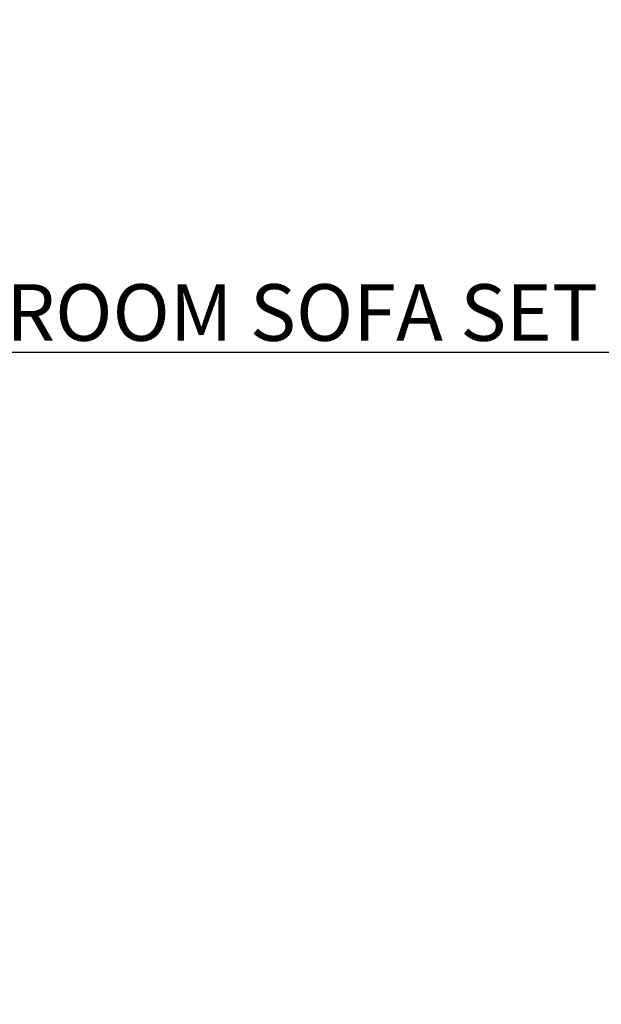
# Model space of a CAD drawing. Units: inches. Extents: x 261 to 2725, y 291 to 1454.
# Tile 18 of 35: x 1043 to 1166, y 644 to 853. Entities that reach past the tile are written whole.
import ezdxf

# ---------------------------------------------------------------- set-up
doc = ezdxf.new("R2010")
doc.units = ezdxf.units.IN
doc.layers.add('A-ANNO-DIMS', color=136, linetype='Continuous', lineweight=18)
doc.styles.get("Standard").update_dxf_attribs({"font": 'arial.ttf'})
doc.dimstyles.new('ISO-25', dxfattribs={"dimtxt": 12, "dimasz": 6, "dimexe": 1.25, "dimexo": 0.625, "dimtad": 1, "dimdec": 0, "dimlunit": 3, "dimtxsty": 'Standard', "dimblk": 'ARCHTICK', "dimcen": 2.5, "dimadec": 0, "dimazin": 0, "dimtfac": 1, "dimtdec": 0, "dimtmove": 0, "dimatfit": 3, "dimfxl": 1, "dimfxlon": 1, "dimarcsym": 0})

# ---------------------------------------------------------------- blocks, each defined once
blk = doc.blocks.new('_ArchTick')
at = {"color": 0, "linetype": 'ByBlock', "const_width": 0.15}
blk.add_lwpolyline([(-0.5, -0.5), (0.5, 0.5)], dxfattribs=at)
blk = doc.blocks.new('*D69')
at = {"layer": 'A-ANNO-DIMS', "color": 0, "lineweight": -2, "ltscale": 0.07, "transparency": 16777216}
for p, q in [((772.63, 783.4), (772.63, 781.15)), ((946.45, 783.4), (946.45, 781.15)), ((772.63, 782.4), (946.45, 782.4)), ((946.45, 782.4), (1224.37, 782.4))]:
    blk.add_line(p, q, dxfattribs=at)
at = {"layer": 'Defpoints', "color": 0, "ltscale": 0.07, "transparency": 16777216}
for p in [(772.63, 808.47), (946.45, 808.47), (946.45, 782.4)]:
    blk.add_point(p, dxfattribs=at)
at = {"layer": 'A-ANNO-DIMS', "color": 0, "lineweight": -2, "ltscale": 0.07, "transparency": 16777216, "xscale": 6, "yscale": 6, "zscale": 6, "rotation": 180}
blk.add_blockref('_ArchTick', (772.63, 782.4), dxfattribs=at)
at = {"layer": 'A-ANNO-DIMS', "color": 0, "lineweight": -2, "ltscale": 0.07, "transparency": 16777216, "xscale": 6, "yscale": 6, "zscale": 6}
blk.add_blockref('_ArchTick', (946.45, 782.4), dxfattribs=at)
at = {"layer": 'A-ANNO-DIMS', "color": 0, "ltscale": 0.07, "transparency": 16777216, "insert": (1088.41, 789.23), "char_height": 12, "attachment_point": 5}
blk.add_mtext('DRAWING ROOM SOFA SET 14\'-6"', dxfattribs=at)
blk = doc.blocks.new('*D82')
at = {"layer": 'A-ANNO-DIMS', "color": 0, "lineweight": -2, "ltscale": 0.07, "transparency": 16777216}
for p, q in [((2600.96, 679.47), (2603.21, 679.47)), ((2601.96, 517.47), (2601.96, 679.47)), ((2600.96, 517.47), (2603.21, 517.47))]:
    blk.add_line(p, q, dxfattribs=at)
at = {"layer": 'Defpoints', "color": 0, "ltscale": 0.07, "transparency": 16777216}
for p in [(946.45, 679.47), (2601.96, 679.47), (946.45, 517.47)]:
    blk.add_point(p, dxfattribs=at)
at = {"layer": 'A-ANNO-DIMS', "color": 0, "lineweight": -2, "ltscale": 0.07, "transparency": 16777216, "xscale": 6, "yscale": 6, "zscale": 6}
for p, rotation in [((2601.96, 679.47), 90), ((2601.96, 517.47), 270)]:
    blk.add_blockref('_ArchTick', p, dxfattribs=dict(at, rotation=rotation))
at = {"layer": 'A-ANNO-DIMS', "color": 0, "ltscale": 0.07, "transparency": 16777216, "insert": (2595.2, 598.47), "char_height": 12, "attachment_point": 5, "rotation": 90}
blk.add_mtext('13\'-6"', dxfattribs=at)
blk = doc.blocks.new('*D83')
at = {"layer": 'A-ANNO-DIMS', "color": 0, "lineweight": -2, "ltscale": 0.07, "transparency": 16777216}
for p, q in [((2600.96, 799.47), (2603.21, 799.47)), ((2601.96, 679.47), (2601.96, 799.47)), ((2600.96, 679.47), (2603.21, 679.47))]:
    blk.add_line(p, q, dxfattribs=at)
at = {"layer": 'Defpoints', "color": 0, "ltscale": 0.07, "transparency": 16777216}
for p in [(946.45, 799.47), (2601.96, 799.47), (946.45, 679.47)]:
    blk.add_point(p, dxfattribs=at)
at = {"layer": 'A-ANNO-DIMS', "color": 0, "lineweight": -2, "ltscale": 0.07, "transparency": 16777216, "xscale": 6, "yscale": 6, "zscale": 6}
for p, rotation in [((2601.96, 799.47), 90), ((2601.96, 679.47), 270)]:
    blk.add_blockref('_ArchTick', p, dxfattribs=dict(at, rotation=rotation))
at = {"layer": 'A-ANNO-DIMS', "color": 0, "ltscale": 0.07, "transparency": 16777216, "insert": (2595.21, 739.47), "char_height": 12, "attachment_point": 5, "rotation": 90}
blk.add_mtext('10\'-0"', dxfattribs=at)
blk = doc.blocks.new('*D84')
at = {"layer": 'A-ANNO-DIMS', "color": 0, "lineweight": -2, "ltscale": 0.07, "transparency": 16777216}
for p, q in [((2600.96, 1024.47), (2603.21, 1024.47)), ((2601.96, 799.47), (2601.96, 1024.47)), ((2600.96, 799.47), (2603.21, 799.47))]:
    blk.add_line(p, q, dxfattribs=at)
at = {"layer": 'Defpoints', "color": 0, "ltscale": 0.07, "transparency": 16777216}
for p in [(946.45, 1024.47), (2601.96, 1024.47), (946.45, 799.47)]:
    blk.add_point(p, dxfattribs=at)
at = {"layer": 'A-ANNO-DIMS', "color": 0, "lineweight": -2, "ltscale": 0.07, "transparency": 16777216, "xscale": 6, "yscale": 6, "zscale": 6}
for p, rotation in [((2601.96, 1024.47), 90), ((2601.96, 799.47), 270)]:
    blk.add_blockref('_ArchTick', p, dxfattribs=dict(at, rotation=rotation))
at = {"layer": 'A-ANNO-DIMS', "color": 0, "ltscale": 0.07, "transparency": 16777216, "insert": (2595.21, 911.97), "char_height": 12, "attachment_point": 5, "rotation": 90}
blk.add_mtext('18\'-9"', dxfattribs=at)
blk = doc.blocks.new('*D103')
at = {"layer": 'A-ANNO-DIMS', "color": 0, "lineweight": -2, "ltscale": 0.07, "transparency": 16777216}
for p, q in [((287.06, 1231.47), (284.81, 1231.47)), ((286.06, 439.47), (286.06, 1231.47)), ((287.06, 439.47), (284.81, 439.47))]:
    blk.add_line(p, q, dxfattribs=at)
at = {"layer": 'Defpoints', "color": 0, "ltscale": 0.07, "transparency": 16777216}
for p in [(286.06, 1231.47), (1243.08, 1231.47), (1243.08, 439.47)]:
    blk.add_point(p, dxfattribs=at)
at = {"layer": 'A-ANNO-DIMS', "color": 0, "lineweight": -2, "ltscale": 0.07, "transparency": 16777216, "xscale": 6, "yscale": 6, "zscale": 6}
for p, rotation in [((286.06, 1231.47), 90), ((286.06, 439.47), 270)]:
    blk.add_blockref('_ArchTick', p, dxfattribs=dict(at, rotation=rotation))
at = {"layer": 'A-ANNO-DIMS', "color": 0, "ltscale": 0.07, "transparency": 16777216, "insert": (279.3, 835.47), "char_height": 12, "attachment_point": 5, "rotation": 90}
blk.add_mtext('66\'-0"', dxfattribs=at)
blk = doc.blocks.new('*D107')
at = {"layer": 'A-ANNO-DIMS', "color": 0, "lineweight": -2, "ltscale": 0.07, "transparency": 16777216}
for p, q in [((287.06, 673.47), (284.81, 673.47)), ((286.06, 496.47), (286.06, 673.47)), ((287.06, 496.47), (284.81, 496.47))]:
    blk.add_line(p, q, dxfattribs=at)
at = {"layer": 'Defpoints', "color": 0, "ltscale": 0.07, "transparency": 16777216}
for p in [(286.06, 673.47), (1252.08, 673.47), (1252.08, 496.47)]:
    blk.add_point(p, dxfattribs=at)
at = {"layer": 'A-ANNO-DIMS', "color": 0, "lineweight": -2, "ltscale": 0.07, "transparency": 16777216, "xscale": 6, "yscale": 6, "zscale": 6}
for p, rotation in [((286.06, 673.47), 90), ((286.06, 496.47), 270)]:
    blk.add_blockref('_ArchTick', p, dxfattribs=dict(at, rotation=rotation))
at = {"layer": 'A-ANNO-DIMS', "color": 0, "ltscale": 0.07, "transparency": 16777216, "insert": (279.3, 584.97), "char_height": 12, "attachment_point": 5, "rotation": 90}
blk.add_mtext('14\'-9"', dxfattribs=at)
blk = doc.blocks.new('*D108')
at = {"layer": 'A-ANNO-DIMS', "color": 0, "lineweight": -2, "ltscale": 0.07, "transparency": 16777216}
for p, q in [((287.06, 799.47), (284.81, 799.47)), ((286.06, 673.47), (286.06, 799.47)), ((287.06, 673.47), (284.81, 673.47))]:
    blk.add_line(p, q, dxfattribs=at)
at = {"layer": 'Defpoints', "color": 0, "ltscale": 0.07, "transparency": 16777216}
for p in [(286.06, 799.47), (1252.08, 799.47), (1252.08, 673.47)]:
    blk.add_point(p, dxfattribs=at)
at = {"layer": 'A-ANNO-DIMS', "color": 0, "lineweight": -2, "ltscale": 0.07, "transparency": 16777216, "xscale": 6, "yscale": 6, "zscale": 6}
for p, rotation in [((286.06, 799.47), 90), ((286.06, 673.47), 270)]:
    blk.add_blockref('_ArchTick', p, dxfattribs=dict(at, rotation=rotation))
at = {"layer": 'A-ANNO-DIMS', "color": 0, "ltscale": 0.07, "transparency": 16777216, "insert": (279.3, 736.47), "char_height": 12, "attachment_point": 5, "rotation": 90}
blk.add_mtext('10\'-6"', dxfattribs=at)
blk = doc.blocks.new('*D109')
at = {"layer": 'A-ANNO-DIMS', "color": 0, "lineweight": -2, "ltscale": 0.07, "transparency": 16777216}
for p, q in [((287.06, 964.47), (284.81, 964.47)), ((286.06, 799.47), (286.06, 964.47)), ((287.06, 799.47), (284.81, 799.47))]:
    blk.add_line(p, q, dxfattribs=at)
at = {"layer": 'Defpoints', "color": 0, "ltscale": 0.07, "transparency": 16777216}
for p in [(286.06, 964.47), (1252.08, 964.47), (1252.08, 799.47)]:
    blk.add_point(p, dxfattribs=at)
at = {"layer": 'A-ANNO-DIMS', "color": 0, "lineweight": -2, "ltscale": 0.07, "transparency": 16777216, "xscale": 6, "yscale": 6, "zscale": 6}
for p, rotation in [((286.06, 964.47), 90), ((286.06, 799.47), 270)]:
    blk.add_blockref('_ArchTick', p, dxfattribs=dict(at, rotation=rotation))
at = {"layer": 'A-ANNO-DIMS', "color": 0, "ltscale": 0.07, "transparency": 16777216, "insert": (279.3, 881.97), "char_height": 12, "attachment_point": 5, "rotation": 90}
blk.add_mtext('13\'-9"', dxfattribs=at)
blk = doc.blocks.new('*D123')
at = {"layer": 'A-ANNO-DIMS', "color": 0, "lineweight": -2, "ltscale": 0.07, "transparency": 16777216}
for p, q in [((287.06, 1054.85), (284.81, 1054.85)), ((286.06, 439.47), (286.06, 1054.85)), ((287.06, 439.47), (284.81, 439.47))]:
    blk.add_line(p, q, dxfattribs=at)
at = {"layer": 'Defpoints', "color": 0, "ltscale": 0.07, "transparency": 16777216}
for p in [(286.06, 1054.85), (2007.71, 1054.85), (2007.71, 439.47)]:
    blk.add_point(p, dxfattribs=at)
at = {"layer": 'A-ANNO-DIMS', "color": 0, "lineweight": -2, "ltscale": 0.07, "transparency": 16777216, "xscale": 6, "yscale": 6, "zscale": 6}
for p, rotation in [((286.06, 1054.85), 90), ((286.06, 439.47), 270)]:
    blk.add_blockref('_ArchTick', p, dxfattribs=dict(at, rotation=rotation))
at = {"layer": 'A-ANNO-DIMS', "color": 0, "ltscale": 0.07, "transparency": 16777216, "insert": (279.22, 747.16), "char_height": 12, "attachment_point": 5, "rotation": 90}
blk.add_mtext('51\'-3 1/2"', dxfattribs=at)

msp = doc.modelspace()

# ---------------------------------------------------------------- dimensions: what is measured, and where the dimension line sits
at = {"layer": 'A-ANNO-DIMS', "ltscale": 0.07}
for base, p1, p2, picture, middle in [((286.06, 1231.47), (1243.08, 439.47), (1243.08, 1231.47), '*D103', (279.3, 835.47)), ((286.06, 1054.85), (2007.71, 439.47), (2007.71, 1054.85), '*D123', (279.22, 747.16)), ((2601.96, 1024.47), (946.45, 799.47), (946.45, 1024.47), '*D84', (2595.21, 911.97)), ((286.06, 964.47), (1252.08, 799.47), (1252.08, 964.47), '*D109', (279.3, 881.97)), ((286.06, 799.47), (1252.08, 673.47), (1252.08, 799.47), '*D108', (279.3, 736.47)), ((2601.96, 799.47), (946.45, 679.47), (946.45, 799.47), '*D83', (2595.21, 739.47)), ((2601.96, 679.47), (946.45, 517.47), (946.45, 679.47), '*D82', (2595.2, 598.47)), ((286.06, 673.47), (1252.08, 496.47), (1252.08, 673.47), '*D107', (279.3, 584.97))]:
    dim = msp.add_linear_dim(base=base, p1=p1, p2=p2, angle=90, dimstyle='ISO-25', override={"dimdec": 1, "dimlfac": 1, "dimrnd": 0, "dimzin": 1, "dimdsep": 46, "dimlunit": 4, "dimfrac": 2}, dxfattribs=at)
    dim.commit()
    dim.dimension.update_dxf_attribs({"geometry": picture, "text_midpoint": middle})
dim = msp.add_linear_dim(base=(946.45, 782.4), p1=(772.63, 808.47), p2=(946.45, 808.47), text='DRAWING ROOM SOFA SET <>', dimstyle='ISO-25', override={"dimdec": 1, "dimrnd": 0, "dimzin": 1, "dimlunit": 4, "dimfrac": 2}, dxfattribs=at)
dim.commit()
dim.dimension.update_dxf_attribs({"geometry": '*D69', "text_midpoint": (1088.41, 789.23)})

doc.saveas('drawing.dxf')
